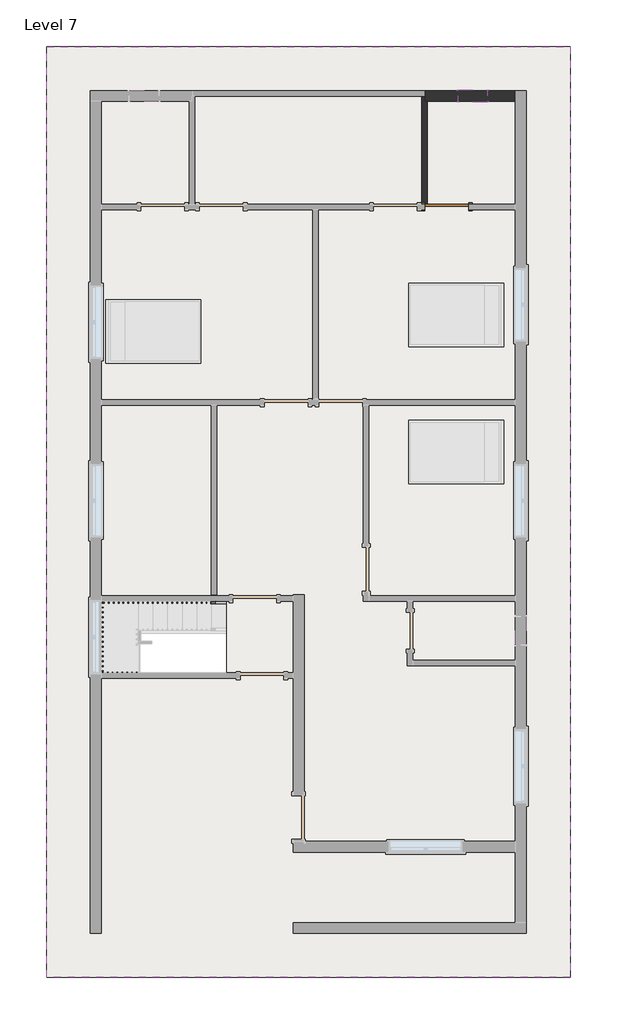
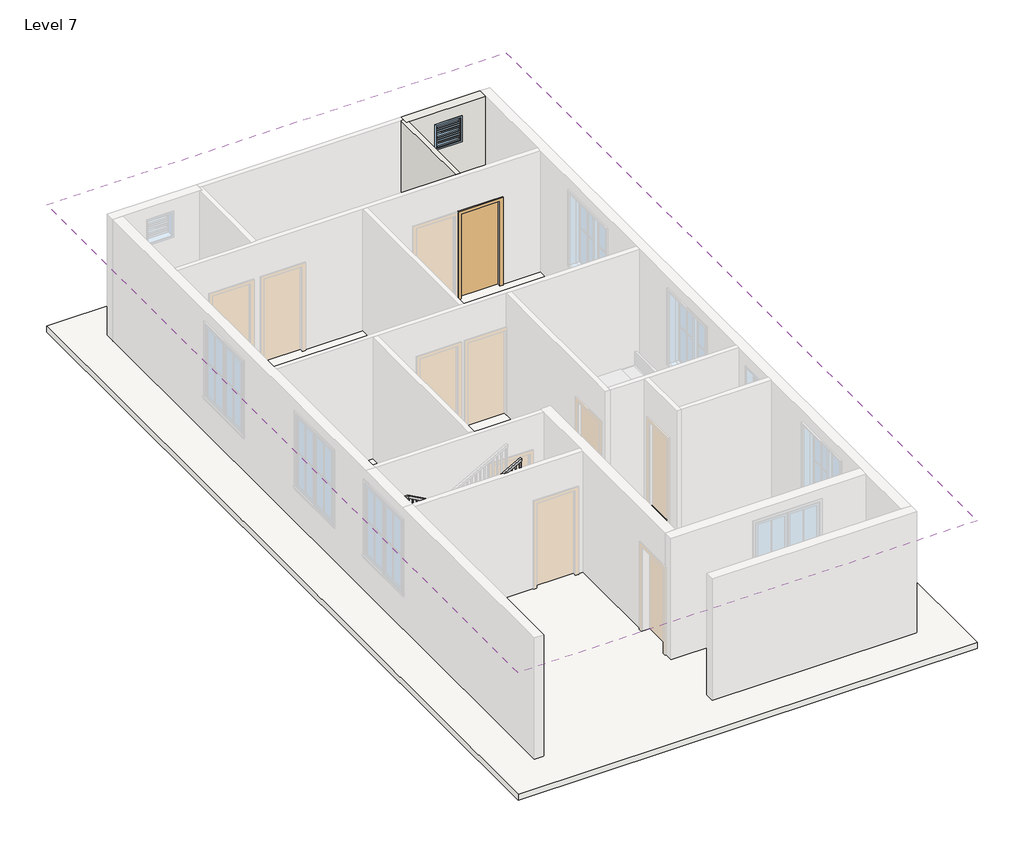
# One storey, part 2 of 3: 2 roofs, 2 walls, 1 door, 1 railing, 1 window.
"""IFC4 building model written with IfcOpenShell, lengths in millimetres."""

from ifc_helpers import new_model, si_unit, frame, origin, place, context, project, spatial, polyline, outline, extrude, faceted_brep, transform, mapped, element, save
from components import single_flush_door_3_305aa2a5, window_f2d8fef0

model = new_model("IFC4")

# Units and contexts
model_context = context("Model", 3, world=origin())
ifc_project = project(units=[si_unit("LENGTHUNIT", "METRE", prefix="MILLI")], contexts=[model_context])

# Site, building, storey
site = spatial("IfcSite", under=ifc_project)
building = spatial("IfcBuilding", under=site)
storey = spatial("IfcBuildingStorey", under=building, Name="Level 7", Elevation=16002.0)

# Door
placement = place(None, origin())
single_flush_door_3_shape = single_flush_door_3_305aa2a5(model_context)
element("IfcDoor", 1, ObjectType="Single-Flush : DOOR 3'", at=placement, inside=storey, context=model_context, shape_type="MappedRepresentation", body=[
    mapped(single_flush_door_3_shape, transform((1622.2379845, 6040.5434309, 16002.0), x_axis=(-1.0, 0.0, 0.0), y_axis=(0.0, -1.0, 0.0), z_axis=(0.0, 0.0, 1.0))),
])

# Railing
element("IfcRailing", 2, ObjectType="Handrail - Rectangular", at=placement, inside=storey, context=model_context, shape_type="SolidModel", body=[
    faceted_brep([(-2968.8120155, -2220.8065691, 17085.7333333), (-2968.8120155, -2220.8065691, 17027.620221), (-2968.8120155, -2170.0065691, 17027.620221), (-2968.8120155, -2170.0065691, 17085.7333333), (-4797.6120155, -2220.8065691, 18101.7333333), (-4810.7756177, -2220.8065691, 18050.9333333), (-4810.7756177, -2170.0065691, 18050.9333333), (-4797.6120155, -2170.0065691, 18101.7333333), (-5508.8120155, -2220.8065691, 18101.7333333), (-5508.8120155, -2220.8065691, 18050.9333333), (-5559.6120155, -2170.0065691, 18050.9333333), (-5559.6120155, -2170.0065691, 18101.7333333), (-5508.8120155, -3624.1565691, 18101.7333333), (-5508.8120155, -3624.1565691, 18050.9333333), (-5559.6120155, -3674.9565691, 18050.9333333), (-5559.6120155, -3674.9565691, 18101.7333333), (-5102.4120155, -3624.1565691, 18101.7333333), (-5089.2484132, -3624.1565691, 18050.9333333), (-5089.2484132, -3674.9565691, 18050.9333333), (-5102.4120155, -3674.9565691, 18101.7333333), (-2968.8120155, -3624.1565691, 19287.0666667), (-2968.8120155, -3674.9565691, 19287.0666667), (-2968.8120155, -3674.9565691, 19228.9535543), (-2968.8120155, -3624.1565691, 19228.9535543)], [[[0, 1, 2, 3]], [[1, 0, 4, 5]], [[2, 1, 5, 6]], [[3, 2, 6, 7]], [[0, 3, 7, 4]], [[5, 4, 8, 9]], [[6, 5, 9, 10]], [[7, 6, 10, 11]], [[4, 7, 11, 8]], [[9, 8, 12, 13]], [[10, 9, 13, 14]], [[11, 10, 14, 15]], [[8, 11, 15, 12]], [[13, 12, 16, 17]], [[14, 13, 17, 18]], [[15, 14, 18, 19]], [[12, 15, 19, 16]], [[20, 21, 22, 23]], [[17, 16, 20, 23]], [[18, 17, 23, 22]], [[19, 18, 22, 21]], [[16, 19, 21, 20]]]),
    extrude(outline(polyline([(19220.1341099, -2984.6870155), (19209.5507765, -3003.7370155), (18203.3333333, -3003.7370155), (18203.3333333, -2984.6870155), (19220.1341099, -2984.6870155)])), frame((0.0, -3659.0815691, 0.0), z_axis=(0.0, 1.0, 0.0), x_axis=(0.0, 0.0, 1.0)), (0.0, 0.0, 1.0), 19.05),
    extrude(outline(polyline([(19163.6896654, -3086.2870155), (19153.1063321, -3105.3370155), (18203.3333333, -3105.3370155), (18203.3333333, -3086.2870155), (19163.6896654, -3086.2870155)])), frame((0.0, -3659.0815691, 0.0), z_axis=(0.0, 1.0, 0.0), x_axis=(0.0, 0.0, 1.0)), (0.0, 0.0, 1.0), 19.05),
    extrude(outline(polyline([(19107.245221, -3187.8870155), (19096.6618876, -3206.9370155), (18203.3333333, -3206.9370155), (18203.3333333, -3187.8870155), (19107.245221, -3187.8870155)])), frame((0.0, -3659.0815691, 0.0), z_axis=(0.0, 1.0, 0.0), x_axis=(0.0, 0.0, 1.0)), (0.0, 0.0, 1.0), 19.05),
    extrude(outline(polyline([(19050.8007765, -3289.4870155), (19040.2174432, -3308.5370155), (18034.0, -3308.5370155), (18034.0, -3289.4870155), (19050.8007765, -3289.4870155)])), frame((0.0, -3659.0815691, 0.0), z_axis=(0.0, 1.0, 0.0), x_axis=(0.0, 0.0, 1.0)), (0.0, 0.0, 1.0), 19.05),
    extrude(outline(polyline([(18994.3563321, -3391.0870155), (18983.7729988, -3410.1370155), (18034.0, -3410.1370155), (18034.0, -3391.0870155), (18994.3563321, -3391.0870155)])), frame((0.0, -3659.0815691, 0.0), z_axis=(0.0, 1.0, 0.0), x_axis=(0.0, 0.0, 1.0)), (0.0, 0.0, 1.0), 19.05),
    extrude(outline(polyline([(18937.9118876, -3492.6870155), (18927.3285543, -3511.7370155), (18034.0, -3511.7370155), (18034.0, -3492.6870155), (18937.9118876, -3492.6870155)])), frame((0.0, -3659.0815691, 0.0), z_axis=(0.0, 1.0, 0.0), x_axis=(0.0, 0.0, 1.0)), (0.0, 0.0, 1.0), 19.05),
    extrude(outline(polyline([(18881.4674432, -3594.2870155), (18870.8841099, -3613.3370155), (17864.6666667, -3613.3370155), (17864.6666667, -3594.2870155), (18881.4674432, -3594.2870155)])), frame((0.0, -3659.0815691, 0.0), z_axis=(0.0, 1.0, 0.0), x_axis=(0.0, 0.0, 1.0)), (0.0, 0.0, 1.0), 19.05),
    extrude(outline(polyline([(18825.0229988, -3695.8870155), (18814.4396654, -3714.9370155), (17864.6666667, -3714.9370155), (17864.6666667, -3695.8870155), (18825.0229988, -3695.8870155)])), frame((0.0, -3659.0815691, 0.0), z_axis=(0.0, 1.0, 0.0), x_axis=(0.0, 0.0, 1.0)), (0.0, 0.0, 1.0), 19.05),
    extrude(outline(polyline([(18768.5785543, -3797.4870155), (18757.995221, -3816.5370155), (17864.6666667, -3816.5370155), (17864.6666667, -3797.4870155), (18768.5785543, -3797.4870155)])), frame((0.0, -3659.0815691, 0.0), z_axis=(0.0, 1.0, 0.0), x_axis=(0.0, 0.0, 1.0)), (0.0, 0.0, 1.0), 19.05),
    extrude(outline(polyline([(18712.1341099, -3899.0870155), (18701.5507765, -3918.1370155), (17695.3333333, -3918.1370155), (17695.3333333, -3899.0870155), (18712.1341099, -3899.0870155)])), frame((0.0, -3659.0815691, 0.0), z_axis=(0.0, 1.0, 0.0), x_axis=(0.0, 0.0, 1.0)), (0.0, 0.0, 1.0), 19.05),
    extrude(outline(polyline([(18655.6896654, -4000.6870155), (18645.1063321, -4019.7370155), (17695.3333333, -4019.7370155), (17695.3333333, -4000.6870155), (18655.6896654, -4000.6870155)])), frame((0.0, -3659.0815691, 0.0), z_axis=(0.0, 1.0, 0.0), x_axis=(0.0, 0.0, 1.0)), (0.0, 0.0, 1.0), 19.05),
    extrude(outline(polyline([(18599.245221, -4102.2870155), (18588.6618876, -4121.3370155), (17695.3333333, -4121.3370155), (17695.3333333, -4102.2870155), (18599.245221, -4102.2870155)])), frame((0.0, -3659.0815691, 0.0), z_axis=(0.0, 1.0, 0.0), x_axis=(0.0, 0.0, 1.0)), (0.0, 0.0, 1.0), 19.05),
    extrude(outline(polyline([(18542.8007765, -4203.8870155), (18532.2174432, -4222.9370155), (17526.0, -4222.9370155), (17526.0, -4203.8870155), (18542.8007765, -4203.8870155)])), frame((0.0, -3659.0815691, 0.0), z_axis=(0.0, 1.0, 0.0), x_axis=(0.0, 0.0, 1.0)), (0.0, 0.0, 1.0), 19.05),
    extrude(outline(polyline([(18486.3563321, -4305.4870155), (18475.7729988, -4324.5370155), (17526.0, -4324.5370155), (17526.0, -4305.4870155), (18486.3563321, -4305.4870155)])), frame((0.0, -3659.0815691, 0.0), z_axis=(0.0, 1.0, 0.0), x_axis=(0.0, 0.0, 1.0)), (0.0, 0.0, 1.0), 19.05),
    extrude(outline(polyline([(18429.9118876, -4407.0870155), (18419.3285543, -4426.1370155), (17526.0, -4426.1370155), (17526.0, -4407.0870155), (18429.9118876, -4407.0870155)])), frame((0.0, -3659.0815691, 0.0), z_axis=(0.0, 1.0, 0.0), x_axis=(0.0, 0.0, 1.0)), (0.0, 0.0, 1.0), 19.05),
    extrude(outline(polyline([(18373.4674432, -4508.6870155), (18362.8841099, -4527.7370155), (17356.6666667, -4527.7370155), (17356.6666667, -4508.6870155), (18373.4674432, -4508.6870155)])), frame((0.0, -3659.0815691, 0.0), z_axis=(0.0, 1.0, 0.0), x_axis=(0.0, 0.0, 1.0)), (0.0, 0.0, 1.0), 19.05),
    extrude(outline(polyline([(18317.0229988, -4610.2870155), (18306.4396654, -4629.3370155), (17356.6666667, -4629.3370155), (17356.6666667, -4610.2870155), (18317.0229988, -4610.2870155)])), frame((0.0, -3659.0815691, 0.0), z_axis=(0.0, 1.0, 0.0), x_axis=(0.0, 0.0, 1.0)), (0.0, 0.0, 1.0), 19.05),
    extrude(outline(polyline([(18260.5785543, -4711.8870155), (18249.995221, -4730.9370155), (17356.6666667, -4730.9370155), (17356.6666667, -4711.8870155), (18260.5785543, -4711.8870155)])), frame((0.0, -3659.0815691, 0.0), z_axis=(0.0, 1.0, 0.0), x_axis=(0.0, 0.0, 1.0)), (0.0, 0.0, 1.0), 19.05),
    extrude(outline(polyline([(18204.1341099, -4813.4870155), (18193.5507765, -4832.5370155), (17187.3333333, -4832.5370155), (17187.3333333, -4813.4870155), (18204.1341099, -4813.4870155)])), frame((0.0, -3659.0815691, 0.0), z_axis=(0.0, 1.0, 0.0), x_axis=(0.0, 0.0, 1.0)), (0.0, 0.0, 1.0), 19.05),
    extrude(outline(polyline([(18147.6896654, -4915.0870155), (18137.1063321, -4934.1370155), (17187.3333333, -4934.1370155), (17187.3333333, -4915.0870155), (18147.6896654, -4915.0870155)])), frame((0.0, -3659.0815691, 0.0), z_axis=(0.0, 1.0, 0.0), x_axis=(0.0, 0.0, 1.0)), (0.0, 0.0, 1.0), 19.05),
    extrude(outline(polyline([(18091.245221, -5016.6870155), (18080.6618876, -5035.7370155), (17187.3333333, -5035.7370155), (17187.3333333, -5016.6870155), (18091.245221, -5016.6870155)])), frame((0.0, -3659.0815691, 0.0), z_axis=(0.0, 1.0, 0.0), x_axis=(0.0, 0.0, 1.0)), (0.0, 0.0, 1.0), 19.05),
    extrude(outline(polyline([(-5137.3370155, -3659.0815691), (-5137.3370155, -3640.0315691), (-5118.2870155, -3640.0315691), (-5118.2870155, -3659.0815691), (-5137.3370155, -3659.0815691)])), frame((0.0, 0.0, 17187.3333333), z_axis=(0.0, 0.0, 1.0), x_axis=(1.0, 0.0, 0.0)), (0.0, 0.0, 1.0), 863.6),
    extrude(outline(polyline([(-5238.9370155, -3659.0815691), (-5238.9370155, -3640.0315691), (-5219.8870155, -3640.0315691), (-5219.8870155, -3659.0815691), (-5238.9370155, -3659.0815691)])), frame((0.0, 0.0, 17187.3333333), z_axis=(0.0, 0.0, 1.0), x_axis=(1.0, 0.0, 0.0)), (0.0, 0.0, 1.0), 863.6),
    extrude(outline(polyline([(-5340.5370155, -3659.0815691), (-5340.5370155, -3640.0315691), (-5321.4870155, -3640.0315691), (-5321.4870155, -3659.0815691), (-5340.5370155, -3659.0815691)])), frame((0.0, 0.0, 17187.3333333), z_axis=(0.0, 0.0, 1.0), x_axis=(1.0, 0.0, 0.0)), (0.0, 0.0, 1.0), 863.6),
    extrude(outline(polyline([(-5442.1370155, -3659.0815691), (-5442.1370155, -3640.0315691), (-5423.0870155, -3640.0315691), (-5423.0870155, -3659.0815691), (-5442.1370155, -3659.0815691)])), frame((0.0, 0.0, 17187.3333333), z_axis=(0.0, 0.0, 1.0), x_axis=(1.0, 0.0, 0.0)), (0.0, 0.0, 1.0), 863.6),
    extrude(outline(polyline([(-5543.7370155, -3608.2815691), (-5524.6870155, -3608.2815691), (-5524.6870155, -3627.3315691), (-5543.7370155, -3627.3315691), (-5543.7370155, -3608.2815691)])), frame((0.0, 0.0, 17187.3333333), z_axis=(0.0, 0.0, 1.0), x_axis=(1.0, 0.0, 0.0)), (0.0, 0.0, 1.0), 863.6),
    extrude(outline(polyline([(-5543.7370155, -3506.6815691), (-5524.6870155, -3506.6815691), (-5524.6870155, -3525.7315691), (-5543.7370155, -3525.7315691), (-5543.7370155, -3506.6815691)])), frame((0.0, 0.0, 17187.3333333), z_axis=(0.0, 0.0, 1.0), x_axis=(1.0, 0.0, 0.0)), (0.0, 0.0, 1.0), 863.6),
    extrude(outline(polyline([(-5543.7370155, -3405.0815691), (-5524.6870155, -3405.0815691), (-5524.6870155, -3424.1315691), (-5543.7370155, -3424.1315691), (-5543.7370155, -3405.0815691)])), frame((0.0, 0.0, 17187.3333333), z_axis=(0.0, 0.0, 1.0), x_axis=(1.0, 0.0, 0.0)), (0.0, 0.0, 1.0), 863.6),
    extrude(outline(polyline([(-5543.7370155, -3303.4815691), (-5524.6870155, -3303.4815691), (-5524.6870155, -3322.5315691), (-5543.7370155, -3322.5315691), (-5543.7370155, -3303.4815691)])), frame((0.0, 0.0, 17187.3333333), z_axis=(0.0, 0.0, 1.0), x_axis=(1.0, 0.0, 0.0)), (0.0, 0.0, 1.0), 863.6),
    extrude(outline(polyline([(-5543.7370155, -3201.8815691), (-5524.6870155, -3201.8815691), (-5524.6870155, -3220.9315691), (-5543.7370155, -3220.9315691), (-5543.7370155, -3201.8815691)])), frame((0.0, 0.0, 17187.3333333), z_axis=(0.0, 0.0, 1.0), x_axis=(1.0, 0.0, 0.0)), (0.0, 0.0, 1.0), 863.6),
    extrude(outline(polyline([(-5543.7370155, -3100.2815691), (-5524.6870155, -3100.2815691), (-5524.6870155, -3119.3315691), (-5543.7370155, -3119.3315691), (-5543.7370155, -3100.2815691)])), frame((0.0, 0.0, 17187.3333333), z_axis=(0.0, 0.0, 1.0), x_axis=(1.0, 0.0, 0.0)), (0.0, 0.0, 1.0), 863.6),
    extrude(outline(polyline([(-5543.7370155, -2998.6815691), (-5524.6870155, -2998.6815691), (-5524.6870155, -3017.7315691), (-5543.7370155, -3017.7315691), (-5543.7370155, -2998.6815691)])), frame((0.0, 0.0, 17187.3333333), z_axis=(0.0, 0.0, 1.0), x_axis=(1.0, 0.0, 0.0)), (0.0, 0.0, 1.0), 863.6),
    extrude(outline(polyline([(-5543.7370155, -2897.0815691), (-5524.6870155, -2897.0815691), (-5524.6870155, -2916.1315691), (-5543.7370155, -2916.1315691), (-5543.7370155, -2897.0815691)])), frame((0.0, 0.0, 17187.3333333), z_axis=(0.0, 0.0, 1.0), x_axis=(1.0, 0.0, 0.0)), (0.0, 0.0, 1.0), 863.6),
    extrude(outline(polyline([(-5543.7370155, -2795.4815691), (-5524.6870155, -2795.4815691), (-5524.6870155, -2814.5315691), (-5543.7370155, -2814.5315691), (-5543.7370155, -2795.4815691)])), frame((0.0, 0.0, 17187.3333333), z_axis=(0.0, 0.0, 1.0), x_axis=(1.0, 0.0, 0.0)), (0.0, 0.0, 1.0), 863.6),
    extrude(outline(polyline([(-5543.7370155, -2693.8815691), (-5524.6870155, -2693.8815691), (-5524.6870155, -2712.9315691), (-5543.7370155, -2712.9315691), (-5543.7370155, -2693.8815691)])), frame((0.0, 0.0, 17187.3333333), z_axis=(0.0, 0.0, 1.0), x_axis=(1.0, 0.0, 0.0)), (0.0, 0.0, 1.0), 863.6),
    extrude(outline(polyline([(-5543.7370155, -2592.2815691), (-5524.6870155, -2592.2815691), (-5524.6870155, -2611.3315691), (-5543.7370155, -2611.3315691), (-5543.7370155, -2592.2815691)])), frame((0.0, 0.0, 17187.3333333), z_axis=(0.0, 0.0, 1.0), x_axis=(1.0, 0.0, 0.0)), (0.0, 0.0, 1.0), 863.6),
    extrude(outline(polyline([(-5543.7370155, -2490.6815691), (-5524.6870155, -2490.6815691), (-5524.6870155, -2509.7315691), (-5543.7370155, -2509.7315691), (-5543.7370155, -2490.6815691)])), frame((0.0, 0.0, 17187.3333333), z_axis=(0.0, 0.0, 1.0), x_axis=(1.0, 0.0, 0.0)), (0.0, 0.0, 1.0), 863.6),
    extrude(outline(polyline([(-5543.7370155, -2389.0815691), (-5524.6870155, -2389.0815691), (-5524.6870155, -2408.1315691), (-5543.7370155, -2408.1315691), (-5543.7370155, -2389.0815691)])), frame((0.0, 0.0, 17187.3333333), z_axis=(0.0, 0.0, 1.0), x_axis=(1.0, 0.0, 0.0)), (0.0, 0.0, 1.0), 863.6),
    extrude(outline(polyline([(-5543.7370155, -2287.4815691), (-5524.6870155, -2287.4815691), (-5524.6870155, -2306.5315691), (-5543.7370155, -2306.5315691), (-5543.7370155, -2287.4815691)])), frame((0.0, 0.0, 17187.3333333), z_axis=(0.0, 0.0, 1.0), x_axis=(1.0, 0.0, 0.0)), (0.0, 0.0, 1.0), 863.6),
    extrude(outline(polyline([(-5499.2870155, -2185.8815691), (-5499.2870155, -2204.9315691), (-5518.3370155, -2204.9315691), (-5518.3370155, -2185.8815691), (-5499.2870155, -2185.8815691)])), frame((0.0, 0.0, 17187.3333333), z_axis=(0.0, 0.0, 1.0), x_axis=(1.0, 0.0, 0.0)), (0.0, 0.0, 1.0), 863.6),
    extrude(outline(polyline([(-5397.6870155, -2185.8815691), (-5397.6870155, -2204.9315691), (-5416.7370155, -2204.9315691), (-5416.7370155, -2185.8815691), (-5397.6870155, -2185.8815691)])), frame((0.0, 0.0, 17187.3333333), z_axis=(0.0, 0.0, 1.0), x_axis=(1.0, 0.0, 0.0)), (0.0, 0.0, 1.0), 863.6),
    extrude(outline(polyline([(-5296.0870155, -2185.8815691), (-5296.0870155, -2204.9315691), (-5315.1370155, -2204.9315691), (-5315.1370155, -2185.8815691), (-5296.0870155, -2185.8815691)])), frame((0.0, 0.0, 17187.3333333), z_axis=(0.0, 0.0, 1.0), x_axis=(1.0, 0.0, 0.0)), (0.0, 0.0, 1.0), 863.6),
    extrude(outline(polyline([(-5194.4870155, -2185.8815691), (-5194.4870155, -2204.9315691), (-5213.5370155, -2204.9315691), (-5213.5370155, -2185.8815691), (-5194.4870155, -2185.8815691)])), frame((0.0, 0.0, 17187.3333333), z_axis=(0.0, 0.0, 1.0), x_axis=(1.0, 0.0, 0.0)), (0.0, 0.0, 1.0), 863.6),
    extrude(outline(polyline([(-5092.8870155, -2185.8815691), (-5092.8870155, -2204.9315691), (-5111.9370155, -2204.9315691), (-5111.9370155, -2185.8815691), (-5092.8870155, -2185.8815691)])), frame((0.0, 0.0, 17187.3333333), z_axis=(0.0, 0.0, 1.0), x_axis=(1.0, 0.0, 0.0)), (0.0, 0.0, 1.0), 863.6),
    extrude(outline(polyline([(-4991.2870155, -2185.8815691), (-4991.2870155, -2204.9315691), (-5010.3370155, -2204.9315691), (-5010.3370155, -2185.8815691), (-4991.2870155, -2185.8815691)])), frame((0.0, 0.0, 17187.3333333), z_axis=(0.0, 0.0, 1.0), x_axis=(1.0, 0.0, 0.0)), (0.0, 0.0, 1.0), 863.6),
    extrude(outline(polyline([(-4889.6870155, -2185.8815691), (-4889.6870155, -2204.9315691), (-4908.7370155, -2204.9315691), (-4908.7370155, -2185.8815691), (-4889.6870155, -2185.8815691)])), frame((0.0, 0.0, 17187.3333333), z_axis=(0.0, 0.0, 1.0), x_axis=(1.0, 0.0, 0.0)), (0.0, 0.0, 1.0), 863.6),
    extrude(outline(polyline([(18038.3285543, -4788.0870155), (18048.9118876, -4807.1370155), (17187.3333333, -4807.1370155), (17187.3333333, -4788.0870155), (18038.3285543, -4788.0870155)])), frame((0.0, -2204.9315691, 0.0), z_axis=(0.0, 1.0, 0.0), x_axis=(0.0, 0.0, 1.0)), (0.0, 0.0, 1.0), 19.05),
    extrude(outline(polyline([(17981.8841099, -4686.4870155), (17992.4674432, -4705.5370155), (17018.0, -4705.5370155), (17018.0, -4686.4870155), (17981.8841099, -4686.4870155)])), frame((0.0, -2204.9315691, 0.0), z_axis=(0.0, 1.0, 0.0), x_axis=(0.0, 0.0, 1.0)), (0.0, 0.0, 1.0), 19.05),
    extrude(outline(polyline([(17925.4396654, -4584.8870155), (17936.0229988, -4603.9370155), (17018.0, -4603.9370155), (17018.0, -4584.8870155), (17925.4396654, -4584.8870155)])), frame((0.0, -2204.9315691, 0.0), z_axis=(0.0, 1.0, 0.0), x_axis=(0.0, 0.0, 1.0)), (0.0, 0.0, 1.0), 19.05),
    extrude(outline(polyline([(17868.995221, -4483.2870155), (17879.5785543, -4502.3370155), (17018.0, -4502.3370155), (17018.0, -4483.2870155), (17868.995221, -4483.2870155)])), frame((0.0, -2204.9315691, 0.0), z_axis=(0.0, 1.0, 0.0), x_axis=(0.0, 0.0, 1.0)), (0.0, 0.0, 1.0), 19.05),
    extrude(outline(polyline([(17812.5507765, -4381.6870155), (17823.1341099, -4400.7370155), (16848.6666667, -4400.7370155), (16848.6666667, -4381.6870155), (17812.5507765, -4381.6870155)])), frame((0.0, -2204.9315691, 0.0), z_axis=(0.0, 1.0, 0.0), x_axis=(0.0, 0.0, 1.0)), (0.0, 0.0, 1.0), 19.05),
    extrude(outline(polyline([(17756.1063321, -4280.0870155), (17766.6896654, -4299.1370155), (16848.6666667, -4299.1370155), (16848.6666667, -4280.0870155), (17756.1063321, -4280.0870155)])), frame((0.0, -2204.9315691, 0.0), z_axis=(0.0, 1.0, 0.0), x_axis=(0.0, 0.0, 1.0)), (0.0, 0.0, 1.0), 19.05),
    extrude(outline(polyline([(17699.6618876, -4178.4870155), (17710.245221, -4197.5370155), (16848.6666667, -4197.5370155), (16848.6666667, -4178.4870155), (17699.6618876, -4178.4870155)])), frame((0.0, -2204.9315691, 0.0), z_axis=(0.0, 1.0, 0.0), x_axis=(0.0, 0.0, 1.0)), (0.0, 0.0, 1.0), 19.05),
    extrude(outline(polyline([(17643.2174432, -4076.8870155), (17653.8007765, -4095.9370155), (16679.3333333, -4095.9370155), (16679.3333333, -4076.8870155), (17643.2174432, -4076.8870155)])), frame((0.0, -2204.9315691, 0.0), z_axis=(0.0, 1.0, 0.0), x_axis=(0.0, 0.0, 1.0)), (0.0, 0.0, 1.0), 19.05),
    extrude(outline(polyline([(17586.7729988, -3975.2870155), (17597.3563321, -3994.3370155), (16679.3333333, -3994.3370155), (16679.3333333, -3975.2870155), (17586.7729988, -3975.2870155)])), frame((0.0, -2204.9315691, 0.0), z_axis=(0.0, 1.0, 0.0), x_axis=(0.0, 0.0, 1.0)), (0.0, 0.0, 1.0), 19.05),
    extrude(outline(polyline([(17530.3285543, -3873.6870155), (17540.9118876, -3892.7370155), (16679.3333333, -3892.7370155), (16679.3333333, -3873.6870155), (17530.3285543, -3873.6870155)])), frame((0.0, -2204.9315691, 0.0), z_axis=(0.0, 1.0, 0.0), x_axis=(0.0, 0.0, 1.0)), (0.0, 0.0, 1.0), 19.05),
    extrude(outline(polyline([(17473.8841099, -3772.0870155), (17484.4674432, -3791.1370155), (16510.0, -3791.1370155), (16510.0, -3772.0870155), (17473.8841099, -3772.0870155)])), frame((0.0, -2204.9315691, 0.0), z_axis=(0.0, 1.0, 0.0), x_axis=(0.0, 0.0, 1.0)), (0.0, 0.0, 1.0), 19.05),
    extrude(outline(polyline([(17417.4396654, -3670.4870155), (17428.0229988, -3689.5370155), (16510.0, -3689.5370155), (16510.0, -3670.4870155), (17417.4396654, -3670.4870155)])), frame((0.0, -2204.9315691, 0.0), z_axis=(0.0, 1.0, 0.0), x_axis=(0.0, 0.0, 1.0)), (0.0, 0.0, 1.0), 19.05),
    extrude(outline(polyline([(17360.995221, -3568.8870155), (17371.5785543, -3587.9370155), (16510.0, -3587.9370155), (16510.0, -3568.8870155), (17360.995221, -3568.8870155)])), frame((0.0, -2204.9315691, 0.0), z_axis=(0.0, 1.0, 0.0), x_axis=(0.0, 0.0, 1.0)), (0.0, 0.0, 1.0), 19.05),
    extrude(outline(polyline([(17304.5507765, -3467.2870155), (17315.1341099, -3486.3370155), (16340.6666667, -3486.3370155), (16340.6666667, -3467.2870155), (17304.5507765, -3467.2870155)])), frame((0.0, -2204.9315691, 0.0), z_axis=(0.0, 1.0, 0.0), x_axis=(0.0, 0.0, 1.0)), (0.0, 0.0, 1.0), 19.05),
    extrude(outline(polyline([(17248.1063321, -3365.6870155), (17258.6896654, -3384.7370155), (16340.6666667, -3384.7370155), (16340.6666667, -3365.6870155), (17248.1063321, -3365.6870155)])), frame((0.0, -2204.9315691, 0.0), z_axis=(0.0, 1.0, 0.0), x_axis=(0.0, 0.0, 1.0)), (0.0, 0.0, 1.0), 19.05),
    extrude(outline(polyline([(17191.6618876, -3264.0870155), (17202.245221, -3283.1370155), (16340.6666667, -3283.1370155), (16340.6666667, -3264.0870155), (17191.6618876, -3264.0870155)])), frame((0.0, -2204.9315691, 0.0), z_axis=(0.0, 1.0, 0.0), x_axis=(0.0, 0.0, 1.0)), (0.0, 0.0, 1.0), 19.05),
    extrude(outline(polyline([(17135.2174432, -3162.4870155), (17145.8007765, -3181.5370155), (16171.3333333, -3181.5370155), (16171.3333333, -3162.4870155), (17135.2174432, -3162.4870155)])), frame((0.0, -2204.9315691, 0.0), z_axis=(0.0, 1.0, 0.0), x_axis=(0.0, 0.0, 1.0)), (0.0, 0.0, 1.0), 19.05),
    extrude(outline(polyline([(17078.7729988, -3060.8870155), (17089.3563321, -3079.9370155), (16171.3333333, -3079.9370155), (16171.3333333, -3060.8870155), (17078.7729988, -3060.8870155)])), frame((0.0, -2204.9315691, 0.0), z_axis=(0.0, 1.0, 0.0), x_axis=(0.0, 0.0, 1.0)), (0.0, 0.0, 1.0), 19.05),
    extrude(outline(polyline([(-5543.7370155, -3640.0315691), (-5524.6870155, -3640.0315691), (-5524.6870155, -3659.0815691), (-5543.7370155, -3659.0815691), (-5543.7370155, -3640.0315691)])), frame((0.0, 0.0, 17187.3333333), z_axis=(0.0, 0.0, 1.0), x_axis=(1.0, 0.0, 0.0)), (0.0, 0.0, 1.0), 863.6),
    extrude(outline(polyline([(-5524.6870155, -2185.8815691), (-5524.6870155, -2204.9315691), (-5543.7370155, -2204.9315691), (-5543.7370155, -2185.8815691), (-5524.6870155, -2185.8815691)])), frame((0.0, 0.0, 17187.3333333), z_axis=(0.0, 0.0, 1.0), x_axis=(1.0, 0.0, 0.0)), (0.0, 0.0, 1.0), 863.6),
    extrude(outline(polyline([(19228.9535543, -2968.8120155), (19218.370221, -2987.8620155), (18203.3333333, -2987.8620155), (18203.3333333, -2968.8120155), (19228.9535543, -2968.8120155)])), frame((0.0, -3659.0815691, 0.0), z_axis=(0.0, 1.0, 0.0), x_axis=(0.0, 0.0, 1.0)), (0.0, 0.0, 1.0), 19.05),
    extrude(outline(polyline([(17027.620221, -2968.8120155), (17038.2035543, -2987.8620155), (16171.3333333, -2987.8620155), (16171.3333333, -2968.8120155), (17027.620221, -2968.8120155)])), frame((0.0, -2204.9315691, 0.0), z_axis=(0.0, 1.0, 0.0), x_axis=(0.0, 0.0, 1.0)), (0.0, 0.0, 1.0), 19.05),
])

# Roofs
element("IfcRoof", 3, ObjectType="ROOF 6\"", at=placement, inside=storey, context=model_context, shape_type="SweptSolid", body=[
    extrude(outline(polyline([(4193.9879845, 9374.2934309), (4193.9879845, -9993.2065691), (-6702.6120155, -9993.2065691), (-6702.6120155, 9374.2934309), (4193.9879845, 9374.2934309)]), holes=[polyline([(-2968.8120155, -2150.9565691), (-5788.2120155, -2150.9565691), (-5788.2120155, -3674.9565691), (-2968.8120155, -3674.9565691), (-2968.8120155, -2150.9565691)])]), frame((0.0, 0.0, 15849.6), z_axis=(0.0, 0.0, 1.0), x_axis=(1.0, 0.0, 0.0)), (0.0, 0.0, 1.0), 152.4),
])
element("IfcRoof", 4, ObjectType="ROOF 6\"", at=placement, inside=storey, context=model_context, shape_type="SweptSolid", body=[
    extrude(outline(polyline([(4193.9879845, 9374.2934309), (4193.9879845, -9993.2065691), (-6702.6120155, -9993.2065691), (-6702.6120155, 9374.2934309), (4193.9879845, 9374.2934309)]), holes=[polyline([(-2968.8120155, -2150.9565691), (-5788.2120155, -2150.9565691), (-5788.2120155, -3674.9565691), (-2968.8120155, -3674.9565691), (-2968.8120155, -2150.9565691)])]), frame((0.0, 0.0, 19050.0), z_axis=(0.0, 0.0, 1.0), x_axis=(1.0, 0.0, 0.0)), (0.0, 0.0, 1.0), 152.4),
])

# Walls
element("IfcWall", 5, ObjectType="WALL 4.5\"", at=placement, inside=storey, context=model_context, shape_type="SweptSolid", body=[
    extrude(outline(polyline([(1107.8879845, 6097.6934309), (1107.8879845, 8345.5934309), (1165.0379845, 8345.5934309), (1165.0379845, 8231.2934309), (1222.1879845, 8231.2934309), (1222.1879845, 6097.6934309), (1107.8879845, 6097.6934309)])), frame((0.0, 0.0, 16002.0), z_axis=(0.0, 0.0, 1.0), x_axis=(1.0, 0.0, 0.0)), (0.0, 0.0, 1.0), 3048.0),
])
element("IfcWall", 6, ObjectType="WALL 9\"", at=placement, inside=storey, context=model_context, shape_type="Brep", body=[
    faceted_brep([(3050.9879845, 8459.8934309, 16002.0), (1165.0379845, 8459.8934309, 16002.0), (1165.0379845, 8459.8934309, 19050.0), (3050.9879845, 8459.8934309, 19050.0), (2469.9629845, 8459.8934309, 18745.2), (1860.3629845, 8459.8934309, 18745.2), (1860.3629845, 8459.8934309, 18135.6), (2469.9629845, 8459.8934309, 18135.6), (3050.9879845, 8231.2934309, 16002.0), (3050.9879845, 8231.2934309, 19050.0), (1222.1879845, 8231.2934309, 19050.0), (1165.0379845, 8231.2934309, 19050.0), (1165.0379845, 8231.2934309, 16002.0), (1222.1879845, 8231.2934309, 16002.0), (2469.9629845, 8231.2934309, 18745.2), (2469.9629845, 8231.2934309, 18135.6), (1860.3629845, 8231.2934309, 18135.6), (1860.3629845, 8231.2934309, 18745.2), (1165.0379845, 8345.5934309, 16002.0), (1165.0379845, 8345.5934309, 19050.0)], [[[0, 1, 2, 3], [4, 5, 6, 7]], [[8, 9, 10, 11, 12, 13], [14, 15, 16, 17]], [[1, 0, 8, 13, 12, 18]], [[2, 1, 18, 12, 11, 19]], [[0, 3, 9, 8]], [[15, 14, 4, 7]], [[16, 15, 7, 6]], [[17, 16, 6, 5]], [[14, 17, 5, 4]], [[3, 2, 19, 11, 10, 9]]]),
])

# Window
window_shape = window_f2d8fef0(model_context)
element("IfcWindow", 7, ObjectType="Window-Louvers : 24\" x 24\"", at=placement, inside=storey, context=model_context, shape_type="MappedRepresentation", body=[
    mapped(window_shape, transform((2165.1629845, 8339.2434309, 17221.2), x_axis=(-1.0, 0.0, 0.0), y_axis=(0.0, -1.0, 0.0), z_axis=(0.0, 0.0, 1.0))),
])

save(model, "model.ifc")

# Revit data of these elements
# Type "Single-Flush : DOOR 3'"
#   Type Mark = "9"
#   Construction Type Id = "MDOOR"
#   Assembly Code = "C1020"
#   Analytic Construction = "Metal"
#   Thickness = 0' - 2"
#   Heat Transfer Coefficient (U) = 0.651978 BTU/(h·ft²·°F)
#   Height = 7' - 0"
#   Trim Projection Ext = 0' - 1"
#   Trim Projection Int = 0' - 1"
#   Trim Width = 0' - 3"
#   Width = 3' - 0"
#   Define Thermal Properties by = 1
#   Door Material = Door - Panel
#   Frame Material = Door - Frame
#   Visual Light Transmittance = 0
#   Solar Heat Gain Coefficient = 0
#   Function = (empty or 0)
#   Wall Closure = (empty or 0)
# Type "Handrail - Rectangular"
#   Assembly Code = "C2010400"
#   built-in parameter 1008612 = 0.0416667 (stored number, unit not read)
#   built-in parameter 1008611 = 0.0416667 (stored number, unit not read)
#   built-in parameter 1008609 = 0.333333 (stored number, unit not read)
#   built-in parameter 1008604 = 0.166667 (stored number, unit not read)
#   built-in parameter 1008603 = 0.166667 (stored number, unit not read)
#   Railing Height = 3' - 0"
#   built-in parameter 1008630 = 2
#   built-in parameter 1008610 = 2
#   built-in parameter 1008618 = Baluster - Square : 3/4"
# Type "ROOF 6\""
#   Assembly Code = "B1020"
#   Layers, outside or top first: 0' - 6" no material (function 1)
# Type "WALL 4.5\""
#   Assembly Code = "B2010"
#   Layers, outside or top first: 0' - 4 1/2" no material (function 1)
# Type "WALL 9\""
#   Assembly Code = "B2010"
#   Layers, outside or top first: 0' - 9" no material (function 1)
# Type "Window-Louvers : 24\" x 24\""
#   Type Mark = "19"
#   Construction Type Id = "GSP4R"
#   Assembly Code = "B20"
#   Analytic Construction = "1/8 in Pilkington single glazing"
#   Visual Light Transmittance = 0.9
#   Thermal Resistance (R) = 1.53941 (h·ft²·°F)/BTU
#   Solar Heat Gain Coefficient = 0.78
#   Max Height = 1' - 11.74264"
#   Height = 2' - 0"
#   Heat Transfer Coefficient (U) = 0.6496 BTU/(h·ft²·°F)
#   Blade Width [instance default] = 1' - 10 1/2"
#   Blade Vertical Thickness = 0' - 0.35355"
#   Blade Thickness = 0' - 0 1/4"
#   Blade Spacing = 0' - 1 1/2"
#   Blade Height = 0' - 1.85355"
#   Blade Depth = 0' - 3"
#   Blade Angle = 45.00°
#   Default Sill Height = 3' - 0"
#   Trim Projection_Exterior = 0' - 0 1/2"
#   Trim Projection_Interior = 0' - 0 1/2"
#   Trim Width_Exterior = 0' - 1 1/2"
#   Trim Width_Interior = 0' - 1 1/2"
#   Width = 2' - 0"
#   Max Blade Count = 12
#   Define Thermal Properties by = 1
#   Blade Count = 12
#   Frame Material = Birch
#   Louver Material = Birch
#   Trim Exterior Material = Birch
#   Trim Interior Material = Birch
#   Wall Closure = (empty or 0)
# Element 1 (IfcDoor, "Single-Flush : DOOR 3'")
#   Phase Created = New Construction
#   Materials on its faces: "Door - Frame", "Door - Panel"
# Element 2 (IfcRailing, "Handrail - Rectangular")
#   Phase Created = New Construction
# Element 3 (IfcRoof, "ROOF 6\"")
#   built-in parameter 1001705 = 52.5 (stored number, unit not read)
#   built-in parameter 1001701 = -0.5 (stored number, unit not read)
#   built-in parameter 1001710 = 33615
#   Phase Created = New Construction
#   Materials on its faces: "Default Roof", "Brick, Common", "Birch"
# Element 4 (IfcRoof, "ROOF 6\"")
#   built-in parameter 1001705 = 63 (stored number, unit not read)
#   built-in parameter 1001701 = 10 (stored number, unit not read)
#   built-in parameter 1001710 = 33615
#   Phase Created = New Construction
#   Materials on its faces: "Default Roof", "Brick, Common", "Birch"
# Element 5 (IfcWall, "WALL 4.5\"")
#   Top Offset = 0' - 0"
#   Base Offset = 0' - 0"
#   Unconnected Height = 10' - 0"
#   wall height = 10' - 0"
#   Phase Created = New Construction
#   Base Constraint = Level 7
#   Materials on its faces: "Default Wall"
# Element 6 (IfcWall, "WALL 9\"")
#   Top Offset = 0' - 0"
#   Base Offset = 0' - 0"
#   Unconnected Height = 10' - 0"
#   wall height = 10' - 0"
#   Phase Created = New Construction
#   Base Constraint = Level 7
#   Materials on its faces: "Default Wall", "Brick, Common"
# Element 7 (IfcWindow, "Window-Louvers : 24\" x 24\"")
#   Mark = "59"
#   Blade Width = 1' - 10 1/2"
#   Phase Created = New Construction
#   Materials on its faces: "Birch"
# Materials
#   "Door - Panel": class "Wood", colour RGB 210 159 95, transparency 0, Cost = 0
#   "Door - Frame": colour RGB 118 70 51, transparency 0, Cost = 0
#   "Birch": class "Wood", colour RGB 224 178 126, transparency 0, Description = "Betula Alleghaniensis", Cost = 0
#   "Default Roof": colour RGB 88 101 114, transparency 0, Cost = 0
#   "Brick, Common": class "Masonry", colour RGB 170 98 104, transparency 0, Description = "Common brick", Cost = 0
#   "Default Wall": colour RGB 128 128 128, transparency 0, Cost = 0
